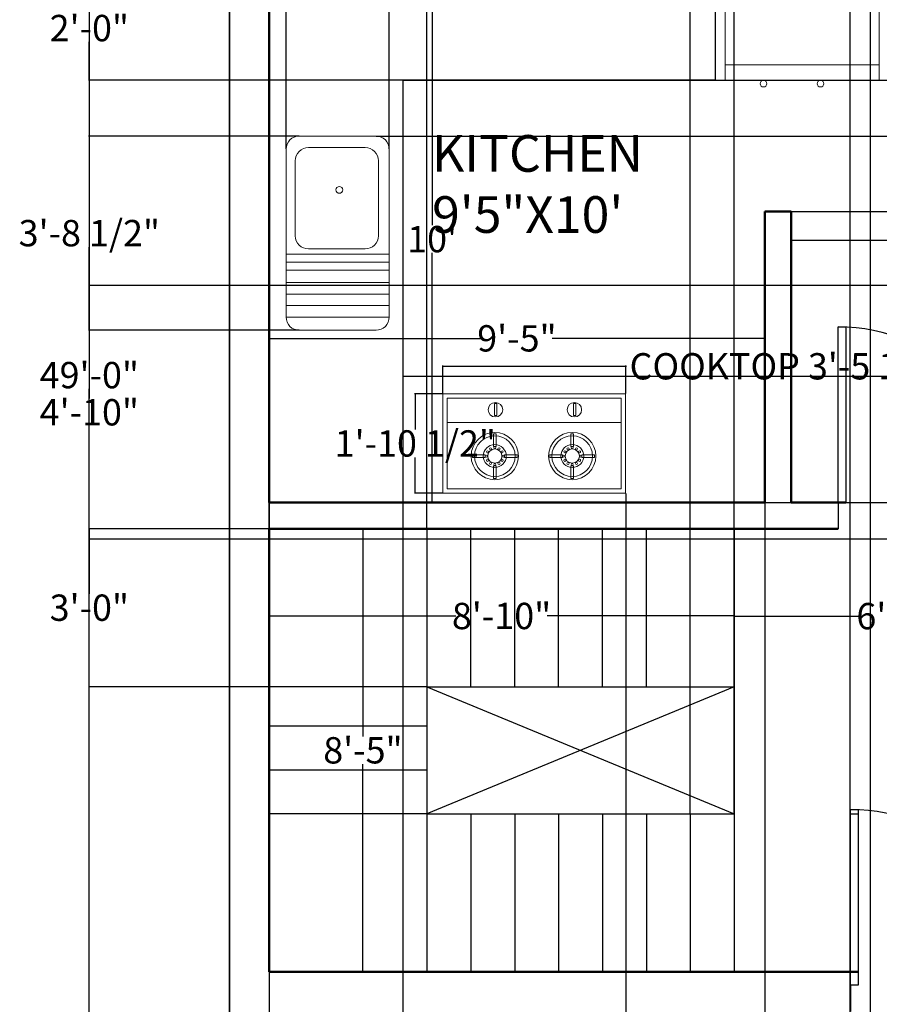
# Model space of a CAD drawing. Units: inches. Extents: x -56 to 545, y -536 to 185.
# Tile 2 of 7: x -54 to 142, y -344 to -120. Entities that reach past the tile are written whole.
import ezdxf

# ---------------------------------------------------------------- set-up
doc = ezdxf.new("R2010")
doc.units = ezdxf.units.IN
doc.header["$MEASUREMENT"] = 0
for name, color, linetype, lineweight in [('A-ANNO-DIMS', 2, 'Continuous', 18), ('A-AREA-IDEN', 4, 'Continuous', 25), ('A-DOOR', 4, 'Continuous', 25), ('A-EQPM', 9, 'Continuous', 18), ('A-FLOR-CASE', 8, 'Continuous', 25), ('A-FLOR-FIXT', 8, 'Continuous', 18), ('A-FLOR-STRS', 7, 'Continuous', 25), ('A-WALL', 7, 'Continuous', 50), ('C-PROP', 7, 'Continuous', 35)]:
    doc.layers.add(name, color=color, linetype=linetype, lineweight=lineweight)
doc.styles.get("Standard").update_dxf_attribs({"font": 'arial.ttf'})
doc.dimstyles.get("Standard").update_dxf_attribs({"dimtxt": 6, "dimasz": 0.18, "dimexe": 0.18, "dimexo": 0.0625, "dimgap": 0.09, "dimtad": 0, "dimtih": 1, "dimtoh": 1, "dimdec": 0, "dimzin": 0, "dimdsep": 46, "dimlunit": 3, "dimtxsty": 'Standard', "dimcen": 0.09, "dimclrd": 3, "dimclre": 3, "dimclrt": 3, "dimadec": 0, "dimazin": 0, "dimtfac": 1, "dimtdec": 0, "dimtofl": 0, "dimtmove": 0, "dimatfit": 3, "dimfxl": 1, "dimtolj": 1, "dimtzin": 0, "dimarcsym": 0})

# ---------------------------------------------------------------- blocks, each defined once
blk = doc.blocks.new('*U7')
for p, q in [((0, 0), (0, -6)), ((40, 0), (40, -6))]:
    blk.add_line(p, q)
blk.add_lwpolyline([(0, 0), (0, 40), (1.75, 40), (1.75, 0)], close=True)
blk.add_arc((0, 0), 40, 0, 90)
blk = doc.blocks.new('A$C06E242FC')
for p, q in [((0, 455.6), (0.5, 456.1)), ((0, 455.6), (0, 0.5)), ((838.9, 456.1), (0.5, 456.1)), ((838.9, 456.1), (839.4, 455.6)), ((839.4, 0.5), (839.4, 455.6)), ((20, 435.6), (20.5, 436.1)), ((20, 435.6), (20, 20.5)), ((818.9, 436.1), (20.5, 436.1)), ((237.3, 411.5), (237.3, 356.2)), ((248.9, 411.5), (237.3, 411.5)), ((248.9, 356.2), (248.9, 411.5)), ((599.3, 411.5), (610.9, 411.5)), ((599.3, 411.5), (599.3, 356.2)), ((610.9, 356.2), (610.9, 411.5)), ((819.4, 435.6), (818.9, 436.1)), ((819.4, 20.5), (819.4, 435.6)), ((20, 324.4), (819.4, 324.4)), ((237.3, 356.2), (248.9, 356.2)), ((599.3, 356.2), (610.9, 356.2)), ((232.7, 272.7), (232.7, 214)), ((244.9, 272.7), (232.7, 272.7)), ((244.9, 214), (244.9, 272.7)), ((588.1, 272.7), (588.1, 214)), ((600.3, 272.7), (588.1, 272.7)), ((600.3, 214), (600.3, 272.7)), ((232.7, 214), (244.9, 214)), ((588.1, 214), (600.3, 214)), ((136.3, 176), (136.3, 163.8)), ((194.9, 176), (136.3, 176)), ((136.3, 163.8), (194.9, 163.8)), ((194.9, 163.8), (194.9, 176)), ((282.9, 176.3), (282.9, 164.1)), ((341.6, 176.3), (282.9, 176.3)), ((282.9, 164.1), (341.6, 164.1)), ((341.6, 164.1), (341.6, 176.3)), ((550.3, 176), (491.7, 176)), ((491.7, 176), (491.7, 163.8)), ((491.7, 163.8), (550.3, 163.8)), ((550.3, 163.8), (550.3, 176)), ((638.3, 176.3), (638.3, 164.1)), ((697, 176.3), (638.3, 176.3)), ((638.3, 164.1), (697, 164.1)), ((697, 164.1), (697, 176.3)), ((245.2, 126.1), (233, 126.1)), ((233, 126.1), (233, 67.4)), ((245.2, 67.4), (245.2, 126.1)), ((600.6, 126.1), (588.3, 126.1)), ((588.3, 126.1), (588.3, 67.4)), ((600.6, 67.4), (600.6, 126.1)), ((233, 67.4), (245.2, 67.4)), ((588.3, 67.4), (600.6, 67.4)), ((0, 0.5), (0.5, 0)), ((20, 20.5), (20.5, 20)), ((20.5, 20), (818.9, 20)), ((818.9, 20), (819.4, 20.5)), ((838.9, 0), (839.4, 0.5)), ((0.5, 0), (838.9, 0))]:
    blk.add_line(p, q)
for centre, radius in [((242, 382.9), 33.3), ((604.1, 382.9), 33.3), ((238.9, 170.1), 108.3), ((594.3, 170.1), 108.3), ((238.9, 170.1), 93.3), ((594.3, 170.1), 93.3), ((238.9, 170.1), 52.6), ((205.3, 189.5), 4.84), ((238.9, 170.1), 32.6), ((219.5, 203.7), 4.84), ((238.9, 208.9), 4.84), ((258.4, 203.7), 4.84), ((272.6, 189.5), 4.84), ((594.3, 170.1), 52.6), ((560.7, 189.5), 4.84), ((594.3, 170.1), 32.6), ((574.9, 203.7), 4.84), ((594.3, 208.9), 4.84), ((613.7, 203.7), 4.84), ((628, 189.5), 4.84), ((200.1, 170.1), 4.84), ((205.3, 150.6), 4.84), ((219.5, 136.4), 4.84), ((238.9, 131.2), 4.84), ((258.4, 136.4), 4.84), ((272.6, 150.6), 4.84), ((277.8, 170.1), 4.84), ((555.5, 170.1), 4.84), ((560.7, 150.6), 4.84), ((574.9, 136.4), 4.84), ((594.3, 131.2), 4.84), ((613.7, 136.4), 4.84), ((628, 150.6), 4.84), ((633.2, 170.1), 4.84)]:
    blk.add_circle(centre, radius)
blk = doc.blocks.new('*D17')
at = {"layer": 'A-ANNO-DIMS', "color": 0, "lineweight": -2, "transparency": 16777216}
for p, q in [((26, -235.84), (24.25, -235.84)), ((24.43, -236.02), (24.43, -283.19)), ((24.43, -336.66), (24.43, -289.49)), ((26, -336.84), (24.25, -336.84))]:
    blk.add_line(p, q, dxfattribs=at)
at = {"layer": 'A-ANNO-DIMS', "color": 0, "transparency": 16777216}
for points in [[(24.4, -236.02), (24.46, -236.02), (24.43, -235.84)], [(24.4, -336.66), (24.46, -336.66), (24.43, -336.84)]]:
    blk.add_solid(points, dxfattribs=at)
at = {"layer": 'Defpoints', "color": 0, "transparency": 16777216}
for p in [(24.43, -235.84), (26.06, -235.84), (26.06, -336.84)]:
    blk.add_point(p, dxfattribs=at)
at = {"layer": 'A-ANNO-DIMS', "color": 0, "transparency": 16777216, "insert": (24.43, -286.34), "char_height": 6, "attachment_point": 5}
blk.add_mtext('\\A1;8\'-5"', dxfattribs=at)
blk = doc.blocks.new('*D18')
at = {"layer": 'A-ANNO-DIMS', "color": 0, "lineweight": -2, "transparency": 16777216}
for p, q in [((3.03, -255.67), (3.03, -255.55)), ((3.21, -255.73), (45.63, -255.73)), ((108.85, -255.73), (66.43, -255.73)), ((109.03, -255.67), (109.03, -255.55))]:
    blk.add_line(p, q, dxfattribs=at)
at = {"layer": 'A-ANNO-DIMS', "color": 0, "transparency": 16777216}
for points in [[(3.21, -255.7), (3.21, -255.76), (3.03, -255.73)], [(108.85, -255.7), (108.85, -255.76), (109.03, -255.73)]]:
    blk.add_solid(points, dxfattribs=at)
at = {"layer": 'Defpoints', "color": 0, "transparency": 16777216}
for p in [(3.03, -255.73), (109.03, -255.73), (109.03, -255.73)]:
    blk.add_point(p, dxfattribs=at)
at = {"layer": 'A-ANNO-DIMS', "color": 0, "transparency": 16777216, "insert": (56.03, -255.73), "char_height": 6, "attachment_point": 5}
blk.add_mtext('\\A1;8\'-10"', dxfattribs=at)
blk = doc.blocks.new('*D19')
at = {"layer": 'A-ANNO-DIMS', "color": 0, "lineweight": -2, "transparency": 16777216}
for p, q in [((108.85, -255.7), (108.85, -255.58)), ((109.03, -255.76), (137.86, -255.76)), ((182.85, -255.76), (154.03, -255.76)), ((183.03, -255.7), (183.03, -255.58))]:
    blk.add_line(p, q, dxfattribs=at)
at = {"layer": 'A-ANNO-DIMS', "color": 0, "transparency": 16777216}
for points in [[(109.03, -255.73), (109.03, -255.79), (108.85, -255.76)], [(182.85, -255.73), (182.85, -255.79), (183.03, -255.76)]]:
    blk.add_solid(points, dxfattribs=at)
at = {"layer": 'Defpoints', "color": 0, "transparency": 16777216}
for p in [(108.85, -255.76), (183.03, -255.76), (183.03, -255.76)]:
    blk.add_point(p, dxfattribs=at)
at = {"layer": 'A-ANNO-DIMS', "color": 0, "transparency": 16777216, "insert": (145.94, -255.76), "char_height": 6, "attachment_point": 5}
blk.add_mtext('\\A1;6\'-2"', dxfattribs=at)
blk = doc.blocks.new('*D20')
at = {"layer": 'A-ANNO-DIMS', "color": 0, "lineweight": -2, "transparency": 16777216}
for p, q in [((96.89, -109.84), (40.02, -109.84)), ((40.2, -110.02), (40.2, -166.69)), ((40.2, -229.66), (40.2, -172.99)), ((96.89, -229.84), (40.02, -229.84))]:
    blk.add_line(p, q, dxfattribs=at)
at = {"layer": 'A-ANNO-DIMS', "color": 0, "transparency": 16777216}
for points in [[(40.17, -110.02), (40.23, -110.02), (40.2, -109.84)], [(40.17, -229.66), (40.23, -229.66), (40.2, -229.84)]]:
    blk.add_solid(points, dxfattribs=at)
at = {"layer": 'Defpoints', "color": 0, "transparency": 16777216}
for p in [(40.2, -109.84), (96.96, -109.84), (96.96, -229.84)]:
    blk.add_point(p, dxfattribs=at)
at = {"layer": 'A-ANNO-DIMS', "color": 0, "transparency": 16777216, "insert": (40.2, -169.84), "char_height": 6, "attachment_point": 5}
blk.add_mtext("\\A1;10'", dxfattribs=at)
blk = doc.blocks.new('*D21')
at = {"layer": 'A-ANNO-DIMS', "color": 0, "lineweight": -2, "transparency": 16777216}
for p, q in [((3.03, -206.65), (3.03, -192.28)), ((3.21, -192.46), (51.47, -192.46)), ((115.85, -192.46), (67.6, -192.46)), ((116.03, -206.65), (116.03, -192.28))]:
    blk.add_line(p, q, dxfattribs=at)
at = {"layer": 'A-ANNO-DIMS', "color": 0, "transparency": 16777216}
for points in [[(3.21, -192.43), (3.21, -192.49), (3.03, -192.46)], [(115.85, -192.43), (115.85, -192.49), (116.03, -192.46)]]:
    blk.add_solid(points, dxfattribs=at)
at = {"layer": 'Defpoints', "color": 0, "transparency": 16777216}
for p in [(116.03, -192.46), (3.03, -206.71), (116.03, -206.71)]:
    blk.add_point(p, dxfattribs=at)
at = {"layer": 'A-ANNO-DIMS', "color": 0, "transparency": 16777216, "insert": (59.53, -192.46), "char_height": 6, "attachment_point": 5}
blk.add_mtext('\\A1;9\'-5"', dxfattribs=at)
blk = doc.blocks.new('*D32')
at = {"layer": 'A-ANNO-DIMS', "color": 0, "lineweight": -2, "transparency": 16777216}
for p, q in [((122.03, -163.65), (122.03, -170.23)), ((345.03, -163.65), (345.03, -170.23)), ((122.21, -170.05), (223.42, -170.05)), ((344.85, -170.05), (243.65, -170.05))]:
    blk.add_line(p, q, dxfattribs=at)
at = {"layer": 'A-ANNO-DIMS', "color": 0, "transparency": 16777216}
for points in [[(122.21, -170.02), (122.21, -170.08), (122.03, -170.05)], [(344.85, -170.02), (344.85, -170.08), (345.03, -170.05)]]:
    blk.add_solid(points, dxfattribs=at)
at = {"layer": 'Defpoints', "color": 0, "transparency": 16777216}
for p in [(122.03, -163.59), (345.03, -163.59), (345.03, -170.05)]:
    blk.add_point(p, dxfattribs=at)
at = {"layer": 'A-ANNO-DIMS', "color": 0, "transparency": 16777216, "insert": (233.53, -170.05), "char_height": 6, "attachment_point": 5}
blk.add_mtext('\\A1;18\'-7"', dxfattribs=at)
blk = doc.blocks.new('*D45')
at = {"layer": 'A-ANNO-DIMS', "color": 3, "lineweight": -2, "transparency": 16777216}
for p, q in [((42.62, -205.02), (42.62, -198.65)), ((42.8, -198.83), (84.14, -198.83)), ((84.32, -205.02), (84.32, -198.65)), ((84.32, -198.83), (84.5, -198.83))]:
    blk.add_line(p, q, dxfattribs=at)
at = {"layer": 'A-ANNO-DIMS', "color": 3, "transparency": 16777216}
for points in [[(42.8, -198.8), (42.8, -198.86), (42.62, -198.83)], [(84.14, -198.8), (84.14, -198.86), (84.32, -198.83)]]:
    blk.add_solid(points, dxfattribs=at)
at = {"layer": 'Defpoints', "color": 0, "transparency": 16777216}
for p in [(84.32, -198.83), (42.62, -205.08), (84.32, -205.08)]:
    blk.add_point(p, dxfattribs=at)
at = {"layer": 'A-ANNO-DIMS', "color": 3, "transparency": 16777216, "insert": (121.64, -198.83), "char_height": 6, "attachment_point": 5}
blk.add_mtext('\\A1;COOKTOP 3\'-5 1/2"', dxfattribs=at)
blk = doc.blocks.new('*D46')
at = {"layer": 'A-ANNO-DIMS', "color": 3, "lineweight": -2, "transparency": 16777216}
for p, q in [((42.56, -205.08), (36.19, -205.08)), ((36.37, -205.26), (36.37, -213.22)), ((36.37, -227.56), (36.37, -219.6)), ((42.56, -227.74), (36.19, -227.74))]:
    blk.add_line(p, q, dxfattribs=at)
at = {"layer": 'A-ANNO-DIMS', "color": 3, "transparency": 16777216}
for points in [[(36.34, -205.26), (36.4, -205.26), (36.37, -205.08)], [(36.34, -227.56), (36.4, -227.56), (36.37, -227.74)]]:
    blk.add_solid(points, dxfattribs=at)
at = {"layer": 'Defpoints', "color": 0, "transparency": 16777216}
for p in [(36.37, -205.08), (42.62, -205.08), (42.62, -227.74)]:
    blk.add_point(p, dxfattribs=at)
at = {"layer": 'A-ANNO-DIMS', "color": 3, "transparency": 16777216, "insert": (36.37, -216.41), "char_height": 6, "attachment_point": 5}
blk.add_mtext('\\A1;1\'-10 1/2"', dxfattribs=at)
blk = doc.blocks.new('*D52')
at = {"layer": 'A-ANNO-DIMS', "color": 3, "lineweight": -2, "transparency": 16777216}
for p, q in [((-6.03, 93.16), (-38.11, 93.16)), ((-37.93, 92.98), (-37.93, -197.69)), ((-37.93, -494.66), (-37.93, -203.99)), ((-6.03, -494.84), (-38.11, -494.84))]:
    blk.add_line(p, q, dxfattribs=at)
at = {"layer": 'A-ANNO-DIMS', "color": 3, "transparency": 16777216}
for points in [[(-37.96, 92.98), (-37.9, 92.98), (-37.93, 93.16)], [(-37.96, -494.66), (-37.9, -494.66), (-37.93, -494.84)]]:
    blk.add_solid(points, dxfattribs=at)
at = {"layer": 'Defpoints', "color": 0, "transparency": 16777216}
for p in [(-5.97, 93.16), (-37.93, -494.84), (-5.97, -494.84)]:
    blk.add_point(p, dxfattribs=at)
at = {"layer": 'A-ANNO-DIMS', "color": 3, "transparency": 16777216, "insert": (-37.93, -200.84), "char_height": 6, "attachment_point": 5}
blk.add_mtext('\\A1;49\'-0"', dxfattribs=at)
blk = doc.blocks.new('*D56')
at = {"layer": 'A-ANNO-DIMS', "color": 3, "lineweight": -2, "transparency": 16777216}
for p, q in [((3.03, -235.78), (3.03, 176.3)), ((3.21, 176.12), (12.97, 176.12)), ((38.85, 176.12), (29.1, 176.12)), ((39.03, -235.78), (39.03, 176.3))]:
    blk.add_line(p, q, dxfattribs=at)
at = {"layer": 'A-ANNO-DIMS', "color": 3, "transparency": 16777216}
for points in [[(3.21, 176.15), (3.21, 176.09), (3.03, 176.12)], [(38.85, 176.15), (38.85, 176.09), (39.03, 176.12)]]:
    blk.add_solid(points, dxfattribs=at)
at = {"layer": 'Defpoints', "color": 0, "transparency": 16777216}
for p in [(39.03, 176.12), (3.03, -235.84), (39.03, -235.84)]:
    blk.add_point(p, dxfattribs=at)
at = {"layer": 'A-ANNO-DIMS', "color": 3, "transparency": 16777216, "insert": (21.03, 176.12), "char_height": 6, "attachment_point": 5}
blk.add_mtext('\\A1;3\'-0"', dxfattribs=at)
blk = doc.blocks.new('*D57')
at = {"layer": 'A-ANNO-DIMS', "color": 3, "lineweight": -2, "transparency": 16777216}
for p, q in [((38.97, -235.84), (-38.11, -235.84)), ((-37.93, -236.02), (-37.93, -250.69)), ((-37.93, -271.66), (-37.93, -257)), ((38.97, -271.84), (-38.11, -271.84))]:
    blk.add_line(p, q, dxfattribs=at)
at = {"layer": 'A-ANNO-DIMS', "color": 3, "transparency": 16777216}
for points in [[(-37.96, -236.02), (-37.9, -236.02), (-37.93, -235.84)], [(-37.96, -271.66), (-37.9, -271.66), (-37.93, -271.84)]]:
    blk.add_solid(points, dxfattribs=at)
at = {"layer": 'Defpoints', "color": 0, "transparency": 16777216}
for p in [(-37.93, -235.84), (39.03, -235.84), (39.03, -271.84)]:
    blk.add_point(p, dxfattribs=at)
at = {"layer": 'A-ANNO-DIMS', "color": 3, "transparency": 16777216, "insert": (-37.93, -253.84), "char_height": 6, "attachment_point": 5}
blk.add_mtext('\\A1;3\'-0"', dxfattribs=at)
blk = doc.blocks.new('*D58')
at = {"layer": 'A-ANNO-DIMS', "color": 3, "lineweight": -2, "transparency": 16777216}
for p, q in [((99.03, -300.78), (99.03, 176.3)), ((99.21, 176.12), (108.85, 176.12)), ((109.03, -300.78), (109.03, 176.3)), ((109.03, 176.12), (109.21, 176.12))]:
    blk.add_line(p, q, dxfattribs=at)
at = {"layer": 'A-ANNO-DIMS', "color": 3, "transparency": 16777216}
for points in [[(99.21, 176.15), (99.21, 176.09), (99.03, 176.12)], [(108.85, 176.15), (108.85, 176.09), (109.03, 176.12)]]:
    blk.add_solid(points, dxfattribs=at)
at = {"layer": 'Defpoints', "color": 0, "transparency": 16777216}
for p in [(109.03, 176.12), (99.03, -300.84), (109.03, -300.84)]:
    blk.add_point(p, dxfattribs=at)
at = {"layer": 'A-ANNO-DIMS', "color": 3, "transparency": 16777216, "insert": (119.61, 176.12), "char_height": 6, "attachment_point": 5}
blk.add_mtext('\\A1;0\'-10"', dxfattribs=at)
blk = doc.blocks.new('*D59')
at = {"layer": 'A-ANNO-DIMS', "color": 3, "lineweight": -2, "transparency": 16777216}
for p, q in [((142.13, -133.66), (530.18, -133.66)), ((530, -133.84), (530, -145.47)), ((530, -163.41), (530, -151.78)), ((122.1, -163.59), (530.18, -163.59))]:
    blk.add_line(p, q, dxfattribs=at)
at = {"layer": 'A-ANNO-DIMS', "color": 3, "transparency": 16777216}
for points in [[(529.97, -133.84), (530.03, -133.84), (530, -133.66)], [(529.97, -163.41), (530.03, -163.41), (530, -163.59)]]:
    blk.add_solid(points, dxfattribs=at)
at = {"layer": 'Defpoints', "color": 0, "transparency": 16777216}
for p in [(142.07, -133.66), (530, -133.66), (122.03, -163.59)]:
    blk.add_point(p, dxfattribs=at)
at = {"layer": 'A-ANNO-DIMS', "color": 3, "transparency": 16777216, "insert": (530, -148.63), "char_height": 6, "attachment_point": 5}
blk.add_mtext('\\A1;2\'-6"', dxfattribs=at)
blk = doc.blocks.new('*D73')
at = {"layer": 'A-ANNO-DIMS', "color": 3, "lineweight": -2, "transparency": 16777216}
for p, q in [((135.38, 28.1), (135.38, -526.99)), ((140.03, 28.1), (140.03, -526.99)), ((135.56, -526.81), (139.85, -526.81)), ((140.03, -526.81), (140.21, -526.81))]:
    blk.add_line(p, q, dxfattribs=at)
at = {"layer": 'A-ANNO-DIMS', "color": 3, "transparency": 16777216}
for points in [[(135.56, -526.78), (135.56, -526.84), (135.38, -526.81)], [(139.85, -526.78), (139.85, -526.84), (140.03, -526.81)]]:
    blk.add_solid(points, dxfattribs=at)
at = {"layer": 'Defpoints', "color": 0, "transparency": 16777216}
for p in [(135.38, 28.16), (140.03, 28.16), (140.03, -526.81)]:
    blk.add_point(p, dxfattribs=at)
at = {"layer": 'A-ANNO-DIMS', "color": 3, "transparency": 16777216, "insert": (155.27, -526.81), "char_height": 6, "attachment_point": 5}
blk.add_mtext('\\A1;0\'-4 1/2"', dxfattribs=at)
blk = doc.blocks.new('*D75')
at = {"layer": 'A-ANNO-DIMS', "color": 3, "lineweight": -2, "transparency": 16777216}
for p, q in [((33.5, -201.14), (33.5, -526.99)), ((3.03, -229.9), (3.03, -526.99)), ((2.85, -526.81), (2.67, -526.81)), ((33.68, -526.81), (33.86, -526.81))]:
    blk.add_line(p, q, dxfattribs=at)
at = {"layer": 'A-ANNO-DIMS', "color": 3, "transparency": 16777216}
for points in [[(2.85, -526.78), (2.85, -526.84), (3.03, -526.81)], [(33.68, -526.78), (33.68, -526.84), (33.5, -526.81)]]:
    blk.add_solid(points, dxfattribs=at)
at = {"layer": 'Defpoints', "color": 0, "transparency": 16777216}
for p in [(33.5, -201.08), (3.03, -229.84), (33.5, -526.81)]:
    blk.add_point(p, dxfattribs=at)
at = {"layer": 'A-ANNO-DIMS', "color": 3, "transparency": 16777216, "insert": (18.27, -526.81), "char_height": 6, "attachment_point": 5}
blk.add_mtext('\\A1;2\'-6 1/2"', dxfattribs=at)
blk = doc.blocks.new('*D76')
at = {"layer": 'A-ANNO-DIMS', "color": 3, "lineweight": -2, "transparency": 16777216}
for p, q in [((2.97, -109.84), (-38.11, -109.84)), ((-37.93, -110.02), (-37.93, -118.6)), ((-37.93, -133.48), (-37.93, -124.91)), ((33.44, -133.66), (-38.11, -133.66))]:
    blk.add_line(p, q, dxfattribs=at)
at = {"layer": 'A-ANNO-DIMS', "color": 3, "transparency": 16777216}
for points in [[(-37.96, -110.02), (-37.9, -110.02), (-37.93, -109.84)], [(-37.96, -133.48), (-37.9, -133.48), (-37.93, -133.66)]]:
    blk.add_solid(points, dxfattribs=at)
at = {"layer": 'Defpoints', "color": 0, "transparency": 16777216}
for p in [(3.03, -109.84), (-37.93, -133.66), (33.5, -133.66)]:
    blk.add_point(p, dxfattribs=at)
at = {"layer": 'A-ANNO-DIMS', "color": 3, "transparency": 16777216, "insert": (-37.93, -121.75), "char_height": 6, "attachment_point": 5}
blk.add_mtext('\\A1;2\'-0"', dxfattribs=at)
blk = doc.blocks.new('*D77')
at = {"layer": 'A-ANNO-DIMS', "color": 3, "lineweight": -2, "transparency": 16777216}
for p, q in [((116.1, -201.08), (530.18, -201.08)), ((530, -201.26), (530, -212.31)), ((530, -229.66), (530, -218.61)), ((116.1, -229.84), (530.18, -229.84))]:
    blk.add_line(p, q, dxfattribs=at)
at = {"layer": 'A-ANNO-DIMS', "color": 3, "transparency": 16777216}
for points in [[(529.97, -201.26), (530.03, -201.26), (530, -201.08)], [(529.97, -229.66), (530.03, -229.66), (530, -229.84)]]:
    blk.add_solid(points, dxfattribs=at)
at = {"layer": 'Defpoints', "color": 0, "transparency": 16777216}
for p in [(116.03, -201.08), (530, -201.08), (116.03, -229.84)]:
    blk.add_point(p, dxfattribs=at)
at = {"layer": 'A-ANNO-DIMS', "color": 3, "transparency": 16777216, "insert": (530, -215.46), "char_height": 6, "attachment_point": 5}
blk.add_mtext('\\A1;2\'-5"', dxfattribs=at)
blk = doc.blocks.new('*D78')
at = {"layer": 'A-ANNO-DIMS', "color": 3, "lineweight": -2, "transparency": 16777216}
for p, q in [((6.93, -149.29), (6.93, 176.3)), ((7.11, 176.12), (30.24, 176.12)), ((30.42, -149.29), (30.42, 176.3)), ((30.42, 176.12), (30.6, 176.12))]:
    blk.add_line(p, q, dxfattribs=at)
at = {"layer": 'A-ANNO-DIMS', "color": 3, "transparency": 16777216}
for points in [[(7.11, 176.15), (7.11, 176.09), (6.93, 176.12)], [(30.24, 176.15), (30.24, 176.09), (30.42, 176.12)]]:
    blk.add_solid(points, dxfattribs=at)
at = {"layer": 'Defpoints', "color": 0, "transparency": 16777216}
for p in [(30.42, 176.12), (6.93, -149.35), (30.42, -149.35)]:
    blk.add_point(p, dxfattribs=at)
at = {"layer": 'A-ANNO-DIMS', "color": 3, "transparency": 16777216, "insert": (47.7, 176.12), "char_height": 6, "attachment_point": 5}
blk.add_mtext('\\A1;1\'-11 1/2"', dxfattribs=at)
blk = doc.blocks.new('*D79')
at = {"layer": 'A-ANNO-DIMS', "color": 3, "lineweight": -2, "transparency": 16777216}
for p, q in [((9.87, -146.35), (-38.11, -146.35)), ((-37.93, -146.53), (-37.93, -165.29)), ((-37.93, -190.43), (-37.93, -171.68)), ((9.87, -190.61), (-38.11, -190.61))]:
    blk.add_line(p, q, dxfattribs=at)
at = {"layer": 'A-ANNO-DIMS', "color": 3, "transparency": 16777216}
for points in [[(-37.96, -146.53), (-37.9, -146.53), (-37.93, -146.35)], [(-37.96, -190.43), (-37.9, -190.43), (-37.93, -190.61)]]:
    blk.add_solid(points, dxfattribs=at)
at = {"layer": 'Defpoints', "color": 0, "transparency": 16777216}
for p in [(9.93, -146.35), (-37.93, -190.61), (9.93, -190.61)]:
    blk.add_point(p, dxfattribs=at)
at = {"layer": 'A-ANNO-DIMS', "color": 3, "transparency": 16777216, "insert": (-37.93, -168.48), "char_height": 6, "attachment_point": 5}
blk.add_mtext('\\A1;3\'-8 1/2"', dxfattribs=at)
blk = doc.blocks.new('*D84')
at = {"layer": 'A-ANNO-DIMS', "color": 3, "lineweight": -2, "transparency": 16777216}
for p, q in [((225.15, -180.41), (-38.11, -180.41)), ((-37.93, -180.59), (-37.93, -206.16)), ((-37.93, -238.04), (-37.93, -212.47)), ((225.15, -238.22), (-38.11, -238.22))]:
    blk.add_line(p, q, dxfattribs=at)
at = {"layer": 'A-ANNO-DIMS', "color": 3, "transparency": 16777216}
for points in [[(-37.96, -180.59), (-37.9, -180.59), (-37.93, -180.41)], [(-37.96, -238.04), (-37.9, -238.04), (-37.93, -238.22)]]:
    blk.add_solid(points, dxfattribs=at)
at = {"layer": 'Defpoints', "color": 0, "transparency": 16777216}
for p in [(225.22, -180.41), (-37.93, -238.22), (225.22, -238.22)]:
    blk.add_point(p, dxfattribs=at)
at = {"layer": 'A-ANNO-DIMS', "color": 3, "transparency": 16777216, "insert": (-37.93, -209.31), "char_height": 6, "attachment_point": 5}
blk.add_mtext('\\A1;4\'-10"', dxfattribs=at)
blk = doc.blocks.new('*D85')
at = {"layer": 'A-ANNO-DIMS', "color": 3, "lineweight": -2, "transparency": 16777216}
for p, q in [((84.32, -227.78), (84.32, -526.99)), ((116.03, -229.9), (116.03, -526.99)), ((84.5, -526.81), (85.07, -526.81)), ((115.85, -526.81), (115.28, -526.81))]:
    blk.add_line(p, q, dxfattribs=at)
at = {"layer": 'A-ANNO-DIMS', "color": 3, "transparency": 16777216}
for points in [[(84.5, -526.78), (84.5, -526.84), (84.32, -526.81)], [(115.85, -526.78), (115.85, -526.84), (116.03, -526.81)]]:
    blk.add_solid(points, dxfattribs=at)
at = {"layer": 'Defpoints', "color": 0, "transparency": 16777216}
for p in [(84.32, -227.71), (116.03, -229.84), (116.03, -526.81)]:
    blk.add_point(p, dxfattribs=at)
at = {"layer": 'A-ANNO-DIMS', "color": 3, "transparency": 16777216, "insert": (100.18, -526.81), "char_height": 6, "attachment_point": 5}
blk.add_mtext('\\A1;2\'-7 1/2"', dxfattribs=at)
blk = doc.blocks.new('*D86')
at = {"layer": 'A-ANNO-DIMS', "color": 3, "lineweight": -2, "transparency": 16777216}
for p, q in [((33.56, -133.66), (530.18, -133.66)), ((530, -133.84), (530, -136.81)), ((530, -146.17), (530, -143.2)), ((27.48, -146.35), (530.18, -146.35))]:
    blk.add_line(p, q, dxfattribs=at)
at = {"layer": 'A-ANNO-DIMS', "color": 3, "transparency": 16777216}
for points in [[(529.97, -133.84), (530.03, -133.84), (530, -133.66)], [(529.97, -146.17), (530.03, -146.17), (530, -146.35)]]:
    blk.add_solid(points, dxfattribs=at)
at = {"layer": 'Defpoints', "color": 0, "transparency": 16777216}
for p in [(33.5, -133.66), (27.42, -146.35), (530, -146.35)]:
    blk.add_point(p, dxfattribs=at)
at = {"layer": 'A-ANNO-DIMS', "color": 3, "transparency": 16777216, "insert": (530, -140.01), "char_height": 6, "attachment_point": 5}
blk.add_mtext('\\A1;1\'-0 1/2"', dxfattribs=at)

msp = doc.modelspace()

# ---------------------------------------------------------------- linework, layer by layer
at = {"layer": 'A-DOOR'}
msp.add_line((135.54, -300.84), (137.29, -300.84), dxfattribs=at)
at = {"layer": 'A-EQPM'}
for p, q in [((107.02, -133.66), (107.02, -109.84)), ((142.07, -109.84), (142.07, -133.66)), ((142.07, -130.14), (107.02, -130.14)), ((142.07, -133.66), (107.02, -133.66))]:
    msp.add_line(p, q, dxfattribs=at)
for centre in [(115.73, -134.42), (128.72, -134.42)]:
    msp.add_circle(centre, 0.755, dxfattribs=at)
at = {"layer": 'A-FLOR-CASE'}
for p, q in [((104.78, -133.66), (104.78, -109.84)), ((104.78, -133.66), (33.5, -133.66)), ((33.5, -133.66), (33.5, -201.08)), ((33.5, -201.08), (116.03, -201.08))]:
    msp.add_line(p, q, dxfattribs=at)
at = {"layer": 'A-FLOR-FIXT'}
for p, q in [((6.93, -173.26), (30.42, -173.26)), ((6.93, -175.1), (30.42, -175.1)), ((6.93, -176.93), (30.42, -176.93)), ((6.93, -179.71), (30.42, -179.71)), ((6.93, -182.39), (30.42, -182.39)), ((6.93, -184.98), (30.42, -184.98)), ((6.93, -187.61), (30.42, -187.61))]:
    msp.add_line(p, q, dxfattribs=at)
for points in [[(9.93, -146.35), (27.42, -146.35, -0.414214), (30.42, -149.35), (30.42, -187.61, -0.414214), (27.42, -190.61), (9.93, -190.61, -0.414214), (6.93, -187.61), (6.93, -149.35, -0.414214)], [(12.02, -149), (24.96, -149, -0.414214), (27.96, -152), (27.96, -169.08, -0.414214), (24.96, -172.08), (12.02, -172.08, -0.414214), (9.02, -169.08), (9.02, -152, -0.414214)]]:
    msp.add_lwpolyline(points, format="xyb", close=True, dxfattribs=at)
msp.add_circle((19.06, -158.64), 0.764, dxfattribs=at)
at = {"layer": 'A-FLOR-STRS'}
for p, q in [((39.03, -235.84), (39.03, -271.84)), ((49.03, -271.84), (49.03, -235.84)), ((59.03, -271.84), (59.03, -235.84)), ((69.03, -271.84), (69.03, -235.84)), ((79.03, -271.84), (79.03, -235.84)), ((89.03, -271.84), (89.03, -235.84)), ((99.03, -271.84), (99.03, -235.84)), ((109.03, -235.84), (109.03, -271.84)), ((39.03, -271.84), (3.03, -271.84)), ((39.03, -271.84), (109.03, -271.84)), ((39.03, -271.84), (39.03, -300.84)), ((39.03, -271.84), (109.03, -300.84)), ((109.03, -271.84), (39.03, -300.84)), ((109.03, -271.84), (109.03, -300.84)), ((39.03, -280.84), (3.03, -280.84)), ((39.03, -290.84), (3.03, -290.84)), ((39.03, -300.84), (3.03, -300.84)), ((39.03, -300.84), (109.03, -300.84)), ((39.03, -300.84), (39.03, -336.84)), ((49.03, -300.84), (49.03, -336.84)), ((59.03, -300.84), (59.03, -336.84)), ((69.03, -300.84), (69.03, -336.84)), ((79.03, -300.84), (79.03, -336.84)), ((89.03, -300.84), (89.03, -336.84)), ((99.03, -300.84), (99.03, -336.84)), ((109.03, -300.84), (109.03, -336.84))]:
    msp.add_line(p, q, dxfattribs=at)
at = {"layer": 'A-WALL'}
for p, q in [((3.03, -109.84), (3.03, -229.84)), ((116.03, -163.59), (116.03, -229.84)), ((116.03, -163.59), (122.03, -163.59)), ((122.03, -163.59), (122.03, -229.84)), ((3.03, -229.84), (116.03, -229.84)), ((122.03, -229.84), (134.51, -229.84)), ((3.03, -235.84), (132.76, -235.84)), ((3.03, -235.84), (3.03, -336.84)), ((3.03, -336.84), (137.29, -336.84))]:
    msp.add_line(p, q, dxfattribs=at)
at = {"layer": 'C-PROP'}
msp.add_line((-5.97, 93.16), (-5.97, -494.84), dxfattribs=at)

# ---------------------------------------------------------------- block references
at = {"layer": 'A-DOOR'}
for p in [(132.76, -229.84), (135.54, -339.84)]:
    msp.add_blockref('*U7', p, dxfattribs=at)
at = {"layer": 'A-EQPM', "xscale": 0.0496756448792194, "yscale": 0.0496756448792194, "zscale": 0.0496756448792194}
msp.add_blockref('A$C06E242FC', (42.62, -227.74), dxfattribs=at)

# ---------------------------------------------------------------- texts
at = {"layer": 'A-AREA-IDEN', "insert": (40.2, -146.14), "char_height": 8.354, "attachment_point": 1}
msp.add_mtext_dynamic_manual_height_columns('{KITCHEN\\P9\'5"X10\'}', width=1091.0728, gutter_width=28.86, heights=[0], dxfattribs=at)

# ---------------------------------------------------------------- dimensions: what is measured, and where the dimension line sits
at = {"layer": 'A-ANNO-DIMS'}
for base, p1, p2, override, picture, middle in [((30.42, 176.12), (6.93, -149.35), (30.42, -149.35), {"dimdec": 1, "dimlfac": 1, "dimrnd": 0, "dimzin": 1, "dimdsep": 46, "dimlunit": 4, "dimfrac": 2}, '*D78', (47.7, 176.12)), ((39.03, 176.12), (3.03, -235.84), (39.03, -235.84), {"dimdec": 1, "dimlfac": 1, "dimrnd": 0, "dimzin": 1, "dimdsep": 46, "dimlunit": 4, "dimfrac": 2}, '*D56', (21.03, 176.12)), ((109.03, 176.12), (99.03, -300.84), (109.03, -300.84), {"dimdec": 1, "dimlfac": 1, "dimrnd": 0, "dimzin": 1, "dimdsep": 46, "dimlunit": 4, "dimfrac": 2}, '*D58', (119.61, 176.12)), ((140.0343, -526.8056), (135.3838, 28.1594), (140.0343, 28.1594), {"dimdec": 1, "dimlfac": 1, "dimrnd": 0, "dimzin": 1, "dimdsep": 46, "dimlunit": 4, "dimfrac": 2}, '*D73', (155.2695, -526.8056)), ((345.03, -170.05), (122.03, -163.59), (345.03, -163.59), {"dimclrd": 0, "dimclre": 0, "dimclrt": 0}, '*D32', (233.53, -170.05)), ((116.03, -192.46), (3.03, -206.71), (116.03, -206.71), {"dimclrd": 0, "dimclre": 0, "dimclrt": 0}, '*D21', (59.53, -192.46)), ((33.5, -526.81), (3.03, -229.84), (33.5, -201.08), {"dimdec": 1, "dimlfac": 1, "dimrnd": 0, "dimzin": 1, "dimdsep": 46, "dimlunit": 4, "dimfrac": 2}, '*D75', (18.27, -526.81)), ((116.03, -526.81), (84.32, -227.71), (116.03, -229.84), {"dimdec": 1, "dimlfac": 1, "dimrnd": 0, "dimzin": 1, "dimdsep": 46, "dimlunit": 4, "dimfrac": 2}, '*D85', (100.18, -526.81)), ((109.03, -255.73), (3.03, -255.73), (109.03, -255.73), {"dimclrd": 0, "dimclre": 0, "dimclrt": 0}, '*D18', (56.03, -255.73)), ((183.03, -255.76), (108.85, -255.76), (183.03, -255.76), {"dimclrd": 0, "dimclre": 0, "dimclrt": 0}, '*D19', (145.94, -255.76))]:
    dim = msp.add_linear_dim(base=base, p1=p1, p2=p2, dimstyle='Standard', override=override, dxfattribs=at)
    dim.commit()
    dim.dimension.update_dxf_attribs({"geometry": picture, "text_midpoint": middle})
for base, p1, p2, override, picture, middle in [((-37.93, -494.84), (-5.97, 93.16), (-5.97, -494.84), {"dimdec": 1, "dimlfac": 1, "dimrnd": 0, "dimzin": 1, "dimdsep": 46, "dimlunit": 4, "dimfrac": 2}, '*D52', (-37.93, -200.84)), ((-37.93, -133.66), (3.03, -109.84), (33.5, -133.66), {"dimdec": 1, "dimlfac": 1, "dimrnd": 0, "dimzin": 1, "dimdsep": 46, "dimlunit": 4, "dimfrac": 2}, '*D76', (-37.93, -121.75)), ((40.2, -109.84), (96.96, -229.84), (96.96, -109.84), {"dimclrd": 0, "dimclre": 0, "dimclrt": 0}, '*D20', (40.2, -169.84)), ((530, -146.35), (33.5, -133.66), (27.42, -146.35), {"dimdec": 1, "dimlfac": 1, "dimrnd": 0, "dimzin": 1, "dimdsep": 46, "dimlunit": 4, "dimfrac": 2}, '*D86', (530, -140.01)), ((530, -133.66), (122.03, -163.59), (142.07, -133.66), {"dimdec": 1, "dimlfac": 1, "dimrnd": 0, "dimzin": 1, "dimdsep": 46, "dimlunit": 4, "dimfrac": 2}, '*D59', (530, -148.63)), ((-37.93, -190.61), (9.93, -146.35), (9.93, -190.61), {"dimdec": 1, "dimlfac": 1, "dimrnd": 0, "dimzin": 1, "dimdsep": 46, "dimlunit": 4, "dimfrac": 2}, '*D79', (-37.93, -168.48)), ((-37.93, -238.22), (225.22, -180.41), (225.22, -238.22), {"dimdec": 1, "dimlfac": 1, "dimrnd": 0, "dimzin": 1, "dimdsep": 46, "dimlunit": 4, "dimfrac": 2}, '*D84', (-37.93, -209.31)), ((530, -201.08), (116.03, -229.84), (116.03, -201.08), {"dimdec": 1, "dimlfac": 1, "dimrnd": 0, "dimzin": 1, "dimdsep": 46, "dimlunit": 4, "dimfrac": 2}, '*D77', (530, -215.46)), ((36.37, -205.08), (42.62, -227.74), (42.62, -205.08), {"dimdec": 1, "dimlfac": 1, "dimrnd": 0, "dimzin": 1, "dimdsep": 46, "dimlunit": 4, "dimfrac": 2}, '*D46', (36.37, -216.41)), ((-37.93, -235.84), (39.03, -271.84), (39.03, -235.84), {"dimdec": 1, "dimlfac": 1, "dimrnd": 0, "dimzin": 1, "dimdsep": 46, "dimlunit": 4, "dimfrac": 2}, '*D57', (-37.93, -253.84)), ((24.43, -235.84), (26.06, -336.84), (26.06, -235.84), {"dimclrd": 0, "dimclre": 0, "dimclrt": 0}, '*D17', (24.43, -286.34))]:
    dim = msp.add_linear_dim(base=base, p1=p1, p2=p2, angle=90, dimstyle='Standard', override=override, dxfattribs=at)
    dim.commit()
    dim.dimension.update_dxf_attribs({"geometry": picture, "text_midpoint": middle})
dim = msp.add_linear_dim(base=(84.32, -198.83), p1=(42.62, -205.08), p2=(84.32, -205.08), text='COOKTOP <>', dimstyle='Standard', override={"dimdec": 1, "dimlfac": 1, "dimrnd": 0, "dimzin": 1, "dimdsep": 46, "dimlunit": 4, "dimfrac": 2}, dxfattribs=at)
dim.commit()
dim.dimension.update_dxf_attribs({"geometry": '*D45', "text_midpoint": (121.64, -198.83)})

doc.saveas('drawing.dxf')
